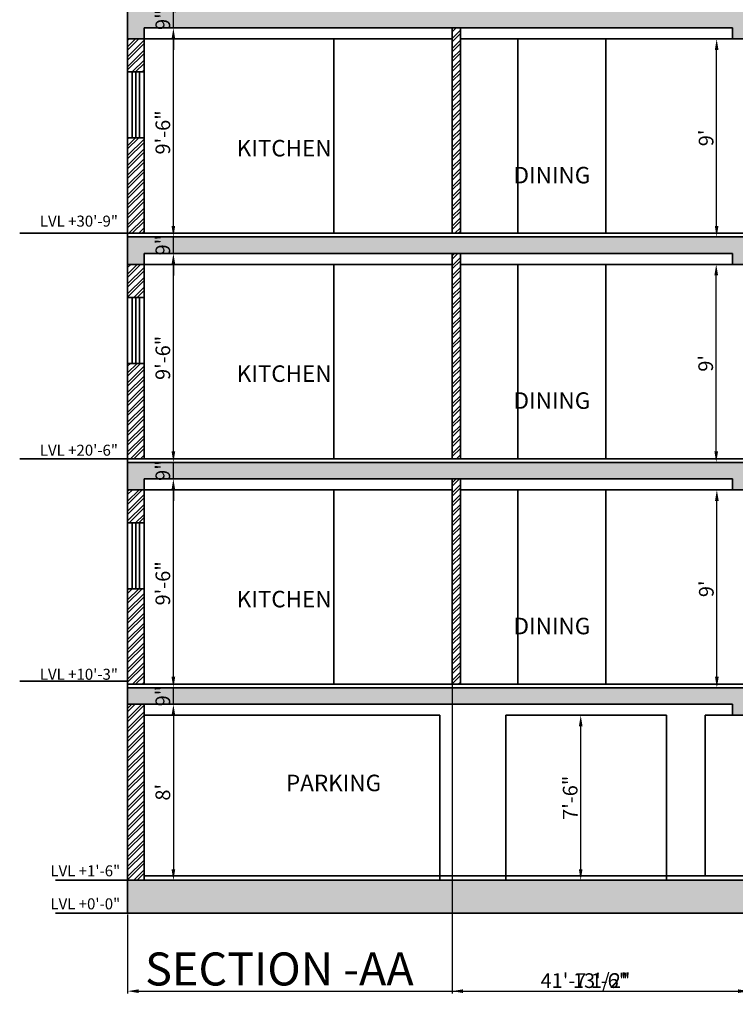
# Model space of a CAD drawing. Units: millimetres. Extents: x 1706 to 5913, y 156 to 1716.
# Tile 18 of 26: x 4417 to 4807, y 156 to 693. Entities that reach past the tile are written whole.
import ezdxf

# ---------------------------------------------------------------- set-up
doc = ezdxf.new("R2010")
doc.units = ezdxf.units.MM
for name, color, linetype, lineweight in [('A-ANNO-DIMS', 2, 'Continuous', 18), ('A-ANNO-SYMB', 3, 'Continuous', 18), ('A-ANNO-TEXT', 7, 'Continuous', 18), ('A-AREA-IDEN', 3, 'Continuous', 18), ('A-SECT', 7, 'Continuous', 35), ('A-SECT-PATT', 8, 'Continuous', 13)]:
    doc.layers.add(name, color=color, linetype=linetype, lineweight=lineweight)
doc.styles.get("Standard").update_dxf_attribs({"font": 'arial.ttf'})
doc.dimstyles.new('ISO-25', dxfattribs={"dimtxt": 8, "dimasz": 6, "dimexe": 1.25, "dimexo": 0.625, "dimtad": 1, "dimdec": 0, "dimlunit": 3, "dimtxsty": 'Standard', "dimcen": 2.5, "dimadec": 0, "dimazin": 0, "dimtfac": 1, "dimtdec": 0, "dimtmove": 0, "dimatfit": 3, "dimfxl": 1, "dimarcsym": 0})
pattern_1 = [(45, (229.4607, 1496.8062), (-2.6940768, 2.6940768), []), (45, (231.2567, 1496.8062), (-2.6940768, 2.6940768), [])]
pattern_2 = [(50, (229.461, 1496.806), (14.574774, -1.275127), [1.524, -16.764]), (355, (229.46, 1496.806), (-2.819474, 15.284548), [1.2192, -13.411247]), (100.45144, (230.675, 1496.7), (11.7553, 14.00942), [1.2952, -14.24722]), (46.1842, (229.46, 1500.87), (21.68632, -3.363386), [2.286, -25.146]), (96.63556, (231.268, 1500.59), (18.99233, 19.79409), [1.9428, -21.37085]), (351.18415, (229.46, 1500.87), (18.99233, 19.79409), [1.8288, -20.11678]), (21, (231.493, 1499.854), (12.12915, -8.181216), [1.524, -16.764]), (326, (231.493, 1499.854), (4.94416, 14.735037), [1.2192, -13.4112]), (71.45144, (232.503, 1499.172), (17.073314, 6.55382), [1.2952, -14.247195]), (37.5, (229.4607, 1496.806), (0.247088, 6.764403), [0, -13.24864, 0, -13.6144, 0, -13.462]), (7.5, (229.461, 1496.806), (5.345573, 8.014446), [0, -7.76224, 0, -12.94384, 0, -5.1308]), (327.5, (224.9293, 1496.806), (10.8472476, -0.4582995), [0, -5.08, 0, -15.8496, 0, -21.0312]), (317.5, (222.897, 1496.806), (11.850335, 2.03412), [0, -6.604, 0, -10.52576, 0, -14.9352])]

# ---------------------------------------------------------------- blocks, each defined once
blk = doc.blocks.new('*D169')
at = {"layer": 'A-ANNO-DIMS', "color": 0, "lineweight": -2, "transparency": 16777216}
for p, q in [((4503.77, 319.75), (4499.62, 319.75)), ((4500.87, 313.75), (4500.87, 229.75)), ((4503.77, 223.75), (4499.62, 223.75))]:
    blk.add_line(p, q, dxfattribs=at)
at = {"layer": 'A-ANNO-DIMS', "color": 0, "transparency": 16777216}
for points in [[(4499.87, 313.75), (4501.87, 313.75), (4500.87, 319.75)], [(4499.87, 229.75), (4501.87, 229.75), (4500.87, 223.75)]]:
    blk.add_solid(points, dxfattribs=at)
at = {"layer": 'Defpoints', "color": 0, "transparency": 16777216}
for p in [(4504.4, 319.75), (4500.87, 223.75), (4504.4, 223.75)]:
    blk.add_point(p, dxfattribs=at)
at = {"layer": 'A-ANNO-DIMS', "color": 0, "transparency": 16777216, "insert": (4496.16, 271.75), "char_height": 8, "attachment_point": 5, "rotation": 90}
blk.add_mtext("8'", dxfattribs=at)
blk = doc.blocks.new('*D170')
at = {"layer": 'A-ANNO-DIMS', "color": 0, "lineweight": -2, "transparency": 16777216}
for p, q in [((4721.21, 313.75), (4724.32, 313.75)), ((4723.07, 229.75), (4723.07, 307.75)), ((4721.21, 223.75), (4724.32, 223.75))]:
    blk.add_line(p, q, dxfattribs=at)
at = {"layer": 'A-ANNO-DIMS', "color": 0, "transparency": 16777216}
for points in [[(4722.07, 307.75), (4724.07, 307.75), (4723.07, 313.75)], [(4722.07, 229.75), (4724.07, 229.75), (4723.07, 223.75)]]:
    blk.add_solid(points, dxfattribs=at)
at = {"layer": 'Defpoints', "color": 0, "transparency": 16777216}
for p in [(4720.58, 313.75), (4723.07, 313.75), (4720.58, 223.75)]:
    blk.add_point(p, dxfattribs=at)
at = {"layer": 'A-ANNO-DIMS', "color": 0, "transparency": 16777216, "insert": (4718.36, 268.75), "char_height": 8, "attachment_point": 5, "rotation": 90}
blk.add_mtext('7\'-6"', dxfattribs=at)
blk = doc.blocks.new('*D171')
at = {"layer": 'A-ANNO-DIMS', "color": 0, "lineweight": -2, "transparency": 16777216}
for p, q in [((4500.87, 334.75), (4500.87, 340.75)), ((4500.87, 319.75), (4500.87, 328.75)), ((4501.49, 328.75), (4502.12, 328.75)), ((4501.49, 319.75), (4502.12, 319.75)), ((4500.87, 313.75), (4500.87, 307.75))]:
    blk.add_line(p, q, dxfattribs=at)
at = {"layer": 'A-ANNO-DIMS', "color": 0, "transparency": 16777216}
for points in [[(4499.87, 334.75), (4501.87, 334.75), (4500.87, 328.75)], [(4499.87, 313.75), (4501.87, 313.75), (4500.87, 319.75)]]:
    blk.add_solid(points, dxfattribs=at)
at = {"layer": 'Defpoints', "color": 0, "transparency": 16777216}
for p in [(4500.87, 328.75), (4500.87, 328.75), (4500.87, 319.75)]:
    blk.add_point(p, dxfattribs=at)
at = {"layer": 'A-ANNO-DIMS', "color": 0, "transparency": 16777216, "insert": (4496.16, 324.25), "char_height": 8, "attachment_point": 5, "rotation": 90}
blk.add_mtext('9"', dxfattribs=at)
blk = doc.blocks.new('*D172')
at = {"layer": 'A-ANNO-DIMS', "color": 0, "lineweight": -2, "transparency": 16777216}
for p, q in [((4501.49, 442.75), (4502.12, 442.75)), ((4500.87, 334.75), (4500.87, 436.75)), ((4501.49, 328.75), (4502.12, 328.75))]:
    blk.add_line(p, q, dxfattribs=at)
at = {"layer": 'A-ANNO-DIMS', "color": 0, "transparency": 16777216}
for points in [[(4499.87, 436.75), (4501.87, 436.75), (4500.87, 442.75)], [(4499.87, 334.75), (4501.87, 334.75), (4500.87, 328.75)]]:
    blk.add_solid(points, dxfattribs=at)
at = {"layer": 'Defpoints', "color": 0, "transparency": 16777216}
for p in [(4500.87, 442.75), (4500.87, 442.75), (4500.87, 328.75)]:
    blk.add_point(p, dxfattribs=at)
at = {"layer": 'A-ANNO-DIMS', "color": 0, "transparency": 16777216, "insert": (4496.16, 385.75), "char_height": 8, "attachment_point": 5, "rotation": 90}
blk.add_mtext('9\'-6"', dxfattribs=at)
blk = doc.blocks.new('*D173')
at = {"layer": 'A-ANNO-DIMS', "color": 0, "lineweight": -2, "transparency": 16777216}
for p, q in [((4500.87, 457.75), (4500.87, 463.75)), ((4500.87, 442.75), (4500.87, 451.75)), ((4501.49, 451.75), (4502.12, 451.75)), ((4501.49, 442.75), (4502.12, 442.75)), ((4500.87, 436.75), (4500.87, 430.75))]:
    blk.add_line(p, q, dxfattribs=at)
at = {"layer": 'A-ANNO-DIMS', "color": 0, "transparency": 16777216}
for points in [[(4499.87, 457.75), (4501.87, 457.75), (4500.87, 451.75)], [(4499.87, 436.75), (4501.87, 436.75), (4500.87, 442.75)]]:
    blk.add_solid(points, dxfattribs=at)
at = {"layer": 'Defpoints', "color": 0, "transparency": 16777216}
for p in [(4500.87, 451.75), (4500.87, 451.75), (4500.87, 442.75)]:
    blk.add_point(p, dxfattribs=at)
at = {"layer": 'A-ANNO-DIMS', "color": 0, "transparency": 16777216, "insert": (4496.16, 447.25), "char_height": 8, "attachment_point": 5, "rotation": 90}
blk.add_mtext('9"', dxfattribs=at)
blk = doc.blocks.new('*D174')
at = {"layer": 'A-ANNO-DIMS', "color": 0, "lineweight": -2, "transparency": 16777216}
for p, q in [((4501.49, 565.75), (4502.12, 565.75)), ((4500.87, 457.75), (4500.87, 559.75)), ((4501.49, 451.75), (4502.12, 451.75))]:
    blk.add_line(p, q, dxfattribs=at)
at = {"layer": 'A-ANNO-DIMS', "color": 0, "transparency": 16777216}
for points in [[(4499.87, 559.75), (4501.87, 559.75), (4500.87, 565.75)], [(4499.87, 457.75), (4501.87, 457.75), (4500.87, 451.75)]]:
    blk.add_solid(points, dxfattribs=at)
at = {"layer": 'Defpoints', "color": 0, "transparency": 16777216}
for p in [(4500.87, 565.75), (4500.87, 565.75), (4500.87, 451.75)]:
    blk.add_point(p, dxfattribs=at)
at = {"layer": 'A-ANNO-DIMS', "color": 0, "transparency": 16777216, "insert": (4496.16, 508.75), "char_height": 8, "attachment_point": 5, "rotation": 90}
blk.add_mtext('9\'-6"', dxfattribs=at)
blk = doc.blocks.new('*D175')
at = {"layer": 'A-ANNO-DIMS', "color": 0, "lineweight": -2, "transparency": 16777216}
for p, q in [((4500.87, 580.75), (4500.87, 586.75)), ((4500.24, 574.75), (4499.62, 574.75)), ((4500.87, 565.75), (4500.87, 574.75)), ((4500.24, 565.75), (4499.62, 565.75)), ((4500.87, 559.75), (4500.87, 553.75))]:
    blk.add_line(p, q, dxfattribs=at)
at = {"layer": 'A-ANNO-DIMS', "color": 0, "transparency": 16777216}
for points in [[(4499.87, 580.75), (4501.87, 580.75), (4500.87, 574.75)], [(4499.87, 559.75), (4501.87, 559.75), (4500.87, 565.75)]]:
    blk.add_solid(points, dxfattribs=at)
at = {"layer": 'Defpoints', "color": 0, "transparency": 16777216}
for p in [(4500.87, 574.75), (4500.87, 574.75), (4500.87, 565.75)]:
    blk.add_point(p, dxfattribs=at)
at = {"layer": 'A-ANNO-DIMS', "color": 0, "transparency": 16777216, "insert": (4496.16, 570.25), "char_height": 8, "attachment_point": 5, "rotation": 90}
blk.add_mtext('9"', dxfattribs=at)
blk = doc.blocks.new('*D176')
at = {"layer": 'A-ANNO-DIMS', "color": 0, "lineweight": -2, "transparency": 16777216}
for p, q in [((4501.49, 688.75), (4502.12, 688.75)), ((4500.87, 580.75), (4500.87, 682.75)), ((4501.49, 574.75), (4502.12, 574.75))]:
    blk.add_line(p, q, dxfattribs=at)
at = {"layer": 'A-ANNO-DIMS', "color": 0, "transparency": 16777216}
for points in [[(4499.87, 682.75), (4501.87, 682.75), (4500.87, 688.75)], [(4499.87, 580.75), (4501.87, 580.75), (4500.87, 574.75)]]:
    blk.add_solid(points, dxfattribs=at)
at = {"layer": 'Defpoints', "color": 0, "transparency": 16777216}
for p in [(4500.87, 688.75), (4500.87, 688.75), (4500.87, 574.75)]:
    blk.add_point(p, dxfattribs=at)
at = {"layer": 'A-ANNO-DIMS', "color": 0, "transparency": 16777216, "insert": (4496.16, 631.75), "char_height": 8, "attachment_point": 5, "rotation": 90}
blk.add_mtext('9\'-6"', dxfattribs=at)
blk = doc.blocks.new('*D177')
at = {"layer": 'A-ANNO-DIMS', "color": 0, "lineweight": -2, "transparency": 16777216}
for p, q in [((4500.87, 703.75), (4500.87, 709.75)), ((4500.87, 688.75), (4500.87, 697.75)), ((4501.49, 697.75), (4502.12, 697.75)), ((4501.49, 688.75), (4502.12, 688.75)), ((4500.87, 682.75), (4500.87, 676.75))]:
    blk.add_line(p, q, dxfattribs=at)
at = {"layer": 'A-ANNO-DIMS', "color": 0, "transparency": 16777216}
for points in [[(4499.87, 703.75), (4501.87, 703.75), (4500.87, 697.75)], [(4499.87, 682.75), (4501.87, 682.75), (4500.87, 688.75)]]:
    blk.add_solid(points, dxfattribs=at)
at = {"layer": 'Defpoints', "color": 0, "transparency": 16777216}
for p in [(4500.87, 697.75), (4500.87, 697.75), (4500.87, 688.75)]:
    blk.add_point(p, dxfattribs=at)
at = {"layer": 'A-ANNO-DIMS', "color": 0, "transparency": 16777216, "insert": (4496.16, 693.25), "char_height": 8, "attachment_point": 5, "rotation": 90}
blk.add_mtext('9"', dxfattribs=at)
blk = doc.blocks.new('*D180')
at = {"layer": 'A-ANNO-DIMS', "color": 0, "lineweight": -2, "transparency": 16777216}
for p, q in [((4800.25, 436.75), (4796.09, 436.75)), ((4797.34, 334.75), (4797.34, 430.75)), ((4800.25, 328.75), (4796.09, 328.75))]:
    blk.add_line(p, q, dxfattribs=at)
at = {"layer": 'A-ANNO-DIMS', "color": 0, "transparency": 16777216}
for points in [[(4796.34, 430.75), (4798.34, 430.75), (4797.34, 436.75)], [(4796.34, 334.75), (4798.34, 334.75), (4797.34, 328.75)]]:
    blk.add_solid(points, dxfattribs=at)
at = {"layer": 'Defpoints', "color": 0, "transparency": 16777216}
for p in [(4797.34, 436.75), (4800.87, 436.75), (4800.87, 328.75)]:
    blk.add_point(p, dxfattribs=at)
at = {"layer": 'A-ANNO-DIMS', "color": 0, "transparency": 16777216, "insert": (4792.63, 382.75), "char_height": 8, "attachment_point": 5, "rotation": 90}
blk.add_mtext("9'", dxfattribs=at)
blk = doc.blocks.new('*D181')
at = {"layer": 'A-ANNO-DIMS', "color": 0, "lineweight": -2, "transparency": 16777216}
for p, q in [((4796.72, 559.75), (4795.74, 559.75)), ((4796.99, 457.75), (4796.99, 553.75)), ((4796.72, 451.75), (4795.74, 451.75))]:
    blk.add_line(p, q, dxfattribs=at)
at = {"layer": 'A-ANNO-DIMS', "color": 0, "transparency": 16777216}
for points in [[(4795.99, 553.75), (4797.99, 553.75), (4796.99, 559.75)], [(4795.99, 457.75), (4797.99, 457.75), (4796.99, 451.75)]]:
    blk.add_solid(points, dxfattribs=at)
at = {"layer": 'Defpoints', "color": 0, "transparency": 16777216}
for p in [(4796.99, 559.75), (4797.34, 559.75), (4797.34, 451.75)]:
    blk.add_point(p, dxfattribs=at)
at = {"layer": 'A-ANNO-DIMS', "color": 0, "transparency": 16777216, "insert": (4792.28, 505.75), "char_height": 8, "attachment_point": 5, "rotation": 90}
blk.add_mtext("9'", dxfattribs=at)
blk = doc.blocks.new('*D182')
at = {"layer": 'A-ANNO-DIMS', "color": 0, "lineweight": -2, "transparency": 16777216}
for p, q in [((4797.62, 682.75), (4798.48, 682.75)), ((4797.23, 580.75), (4797.23, 676.75)), ((4797.62, 574.75), (4798.48, 574.75))]:
    blk.add_line(p, q, dxfattribs=at)
at = {"layer": 'A-ANNO-DIMS', "color": 0, "transparency": 16777216}
for points in [[(4796.23, 676.75), (4798.23, 676.75), (4797.23, 682.75)], [(4796.23, 580.75), (4798.23, 580.75), (4797.23, 574.75)]]:
    blk.add_solid(points, dxfattribs=at)
at = {"layer": 'Defpoints', "color": 0, "transparency": 16777216}
for p in [(4796.99, 682.75), (4797.23, 682.75), (4796.99, 574.75)]:
    blk.add_point(p, dxfattribs=at)
at = {"layer": 'A-ANNO-DIMS', "color": 0, "transparency": 16777216, "insert": (4792.52, 628.75), "char_height": 8, "attachment_point": 5, "rotation": 90}
blk.add_mtext("9'", dxfattribs=at)
blk = doc.blocks.new('*D250')
at = {"layer": 'A-ANNO-DIMS', "color": 0, "lineweight": -2, "transparency": 16777216}
for p, q in [((4475.91, 205.12), (4475.91, 162)), ((4975.41, 205.12), (4975.41, 162)), ((4481.91, 163.25), (4969.41, 163.25))]:
    blk.add_line(p, q, dxfattribs=at)
at = {"layer": 'A-ANNO-DIMS', "color": 0, "transparency": 16777216}
for points in [[(4481.91, 164.25), (4481.91, 162.25), (4475.91, 163.25)], [(4969.41, 164.25), (4969.41, 162.25), (4975.41, 163.25)]]:
    blk.add_solid(points, dxfattribs=at)
at = {"layer": 'Defpoints', "color": 0, "transparency": 16777216}
for p in [(4475.91, 205.75), (4975.41, 205.75), (4975.41, 163.25)]:
    blk.add_point(p, dxfattribs=at)
at = {"layer": 'A-ANNO-DIMS', "color": 0, "transparency": 16777216, "insert": (4725.66, 168.01), "char_height": 8, "attachment_point": 5}
blk.add_mtext('41\'-7 1/2"', dxfattribs=at)
blk = doc.blocks.new('*D254')
at = {"layer": 'A-ANNO-DIMS', "color": 0, "lineweight": -2, "transparency": 16777216}
for p, q in [((4652.91, 330.12), (4652.91, 162)), ((4814.91, 225.62), (4814.91, 162)), ((4658.91, 163.25), (4808.91, 163.25))]:
    blk.add_line(p, q, dxfattribs=at)
at = {"layer": 'A-ANNO-DIMS', "color": 0, "transparency": 16777216}
for points in [[(4658.91, 164.25), (4658.91, 162.25), (4652.91, 163.25)], [(4808.91, 164.25), (4808.91, 162.25), (4814.91, 163.25)]]:
    blk.add_solid(points, dxfattribs=at)
at = {"layer": 'Defpoints', "color": 0, "transparency": 16777216}
for p in [(4652.91, 330.75), (4814.91, 226.25), (4814.91, 163.25)]:
    blk.add_point(p, dxfattribs=at)
at = {"layer": 'A-ANNO-DIMS', "color": 0, "transparency": 16777216, "insert": (4733.91, 167.96), "char_height": 8, "attachment_point": 5}
blk.add_mtext('13\'-6"', dxfattribs=at)

msp = doc.modelspace()

# ---------------------------------------------------------------- hatches: boundary and pattern name
at = {"layer": 'A-SECT-PATT'}
h = msp.add_hatch(dxfattribs=at)
h.set_pattern_fill('AR-CONC', color=256, scale=0.08)
h.set_pattern_definition(pattern_2)
h.paths.add_polyline_path([(4853.91, 697.75), (4475.91, 697.75), (4475.91, 682.75), (4484.91, 682.75), (4484.91, 688.75), (4805.91, 688.75), (4805.91, 682.75), (4822.41, 682.75), (4822.41, 688.75), (4839.28, 688.75), (4927.41, 634.19), (4927.41, 634.75), (4966.41, 634.75), (4966.41, 632.75), (4975.41, 632.75), (4975.41, 641.25), (4927.41, 641.25), (4927.41, 647.75), (4916.91, 647.75), (4916.91, 654.25), (4906.41, 654.25), (4906.41, 660.75), (4895.91, 660.75), (4895.91, 667.25), (4885.41, 667.25), (4885.41, 673.75), (4874.91, 673.75), (4874.91, 680.25), (4864.41, 680.25), (4864.41, 686.75), (4853.91, 686.75)])
h = msp.add_hatch(dxfattribs=at)
h.set_pattern_fill('ANSI32', color=256, scale=0.4)
h.set_pattern_definition(pattern_1)
h.paths.add_polyline_path([(4657.41, 688.75), (4652.91, 688.75), (4652.91, 576.75), (4657.41, 576.75)])
h = msp.add_hatch(dxfattribs=at)
h.set_pattern_fill('ANSI32', color=256, scale=0.4)
h.set_pattern_definition(pattern_1)
h.paths.add_polyline_path([(4484.91, 682.75), (4475.91, 682.75), (4475.91, 664.75), (4484.91, 664.75)])
h = msp.add_hatch(dxfattribs=at)
h.set_pattern_fill('ANSI32', color=256, scale=0.4)
h.set_pattern_definition(pattern_1)
h.paths.add_polyline_path([(4484.91, 628.75), (4475.91, 628.75), (4475.91, 576.75), (4484.91, 576.75)])
h = msp.add_hatch(dxfattribs=at)
h.set_pattern_fill('AR-CONC', color=256, scale=0.08)
h.set_pattern_definition(pattern_2)
h.paths.add_polyline_path([(4853.91, 569.75), (4853.91, 574.75), (4475.91, 574.75), (4475.91, 559.75), (4484.91, 559.75), (4484.91, 565.75), (4805.91, 565.75), (4805.91, 559.75), (4822.41, 559.75), (4822.41, 565.75), (4838.47, 565.75), (4927.41, 510.69), (4927.41, 511.75), (4966.41, 511.75), (4966.41, 509.75), (4975.41, 509.75), (4975.41, 517.75), (4927.41, 517.75), (4927.41, 524.25), (4916.91, 524.25), (4916.91, 530.75), (4906.41, 530.75), (4906.41, 537.25), (4895.91, 537.25), (4895.91, 543.75), (4885.41, 543.75), (4885.41, 550.25), (4874.91, 550.25), (4874.91, 556.75), (4864.41, 556.75), (4864.41, 563.25), (4853.91, 563.25)])
h = msp.add_hatch(dxfattribs=at)
h.set_pattern_fill('ANSI32', color=256, scale=0.4)
h.set_pattern_definition(pattern_1)
h.paths.add_polyline_path([(4657.41, 565.75), (4652.91, 565.75), (4652.91, 453.75), (4657.41, 453.75)])
h = msp.add_hatch(dxfattribs=at)
h.set_pattern_fill('ANSI32', color=256, scale=0.4)
h.set_pattern_definition(pattern_1)
h.paths.add_polyline_path([(4484.91, 559.75), (4475.91, 559.75), (4475.91, 541.75), (4484.91, 541.75)])
h = msp.add_hatch(dxfattribs=at)
h.set_pattern_fill('ANSI32', color=256, scale=0.4)
h.set_pattern_definition(pattern_1)
h.paths.add_polyline_path([(4484.91, 505.75), (4475.91, 505.75), (4475.91, 453.75), (4484.91, 453.75)], flags=17)
h = msp.add_hatch(dxfattribs=at)
h.set_pattern_fill('AR-CONC', color=256, scale=0.08)
h.set_pattern_definition(pattern_2)
h.paths.add_polyline_path([(4853.91, 451.75), (4475.91, 451.75), (4475.91, 436.75), (4484.91, 436.75), (4484.91, 442.75), (4805.91, 442.75), (4805.91, 436.75), (4822.41, 436.75), (4822.41, 442.75), (4842.6, 442.75), (4927.41, 390.25), (4966.41, 390.25), (4966.41, 388.25), (4975.41, 388.25), (4975.41, 396.25), (4927.41, 396.25), (4927.41, 402.75), (4916.91, 402.75), (4916.91, 409.25), (4906.41, 409.25), (4906.41, 415.75), (4895.91, 415.75), (4895.91, 422.25), (4885.41, 422.25), (4885.41, 428.75), (4874.91, 428.75), (4874.91, 435.25), (4864.41, 435.25), (4864.41, 441.75), (4853.91, 441.75)])
h = msp.add_hatch(dxfattribs=at)
h.set_pattern_fill('ANSI32', color=256, scale=0.4)
h.set_pattern_definition(pattern_1)
h.paths.add_polyline_path([(4657.41, 442.75), (4652.91, 442.75), (4652.91, 330.75), (4657.41, 330.75)])
h = msp.add_hatch(dxfattribs=at)
h.set_pattern_fill('ANSI32', color=256, scale=0.4)
h.set_pattern_definition(pattern_1)
h.paths.add_polyline_path([(4484.91, 436.75), (4475.91, 436.75), (4475.91, 418.75), (4484.91, 418.75)])
h = msp.add_hatch(dxfattribs=at)
h.set_pattern_fill('ANSI32', color=256, scale=0.4)
h.set_pattern_definition(pattern_1)
h.paths.add_polyline_path([(4484.91, 382.75), (4475.91, 382.75), (4475.91, 330.75), (4484.91, 330.75)])
h = msp.add_hatch(dxfattribs=at)
h.set_pattern_fill('AR-CONC', color=256, scale=0.08)
h.set_pattern_definition(pattern_2)
h.paths.add_polyline_path([(4864.41, 323.25), (4853.91, 323.25), (4853.91, 328.75), (4475.91, 328.75), (4475.91, 319.75), (4805.91, 319.75), (4805.91, 313.75), (4814.91, 313.75), (4822.41, 313.75), (4822.41, 319.75), (4850.55, 319.75), (4927.41, 271.75), (4969.41, 271.75), (4969.41, 269.75), (4975.41, 269.75), (4975.41, 277.75), (4927.41, 277.75), (4927.41, 284.25), (4916.91, 284.25), (4916.91, 290.75), (4906.41, 290.75), (4906.41, 297.25), (4895.91, 297.25), (4895.91, 303.75), (4885.41, 303.75), (4885.41, 310.25), (4874.91, 310.25), (4874.91, 316.75), (4864.41, 316.75)])
h = msp.add_hatch(dxfattribs=at)
h.set_pattern_fill('ANSI32', color=256, scale=0.4)
h.set_pattern_definition(pattern_1)
h.paths.add_polyline_path([(4484.91, 319.75), (4475.91, 319.75), (4475.91, 223.75), (4484.91, 223.75)])
h = msp.add_hatch(dxfattribs=at)
h.set_pattern_fill('AR-CONC', color=256, scale=0.08)
h.set_pattern_definition(pattern_2)
h.paths.add_polyline_path([(4975.41, 223.75), (4475.91, 223.75), (4475.91, 205.75), (4975.41, 205.75)])

# ---------------------------------------------------------------- linework, layer by layer
at = {"layer": 'A-SECT'}
for p, q in [((4475.91, 856.75), (4475.91, 205.75)), ((4484.91, 688.75), (4484.91, 576.75)), ((4484.91, 688.75), (4805.91, 688.75)), ((4652.91, 688.75), (4652.91, 576.75)), ((4657.41, 688.75), (4657.41, 576.75)), ((4805.91, 682.75), (4805.91, 688.75)), ((4475.91, 682.75), (4652.91, 682.75)), ((4588.41, 682.75), (4588.41, 576.75)), ((4657.41, 682.75), (4822.41, 682.75)), ((4688.69, 576.75), (4688.69, 682.75)), ((4736.69, 576.75), (4736.69, 682.75)), ((4475.91, 664.75), (4484.91, 664.75)), ((4478.41, 664.75), (4478.41, 628.75)), ((4480.41, 664.75), (4480.41, 628.75)), ((4482.41, 664.75), (4482.41, 628.75)), ((4475.91, 628.75), (4484.91, 628.75)), ((4475.91, 576.75), (4417.04, 576.75)), ((4475.91, 574.75), (4853.91, 574.75)), ((4484.91, 565.75), (4484.91, 453.75)), ((4484.91, 565.75), (4805.91, 565.75)), ((4652.91, 565.75), (4652.91, 453.75)), ((4657.41, 565.75), (4657.41, 453.75)), ((4805.91, 559.75), (4805.91, 565.75)), ((4475.91, 559.75), (4652.91, 559.75)), ((4588.41, 559.75), (4588.41, 453.75)), ((4657.41, 559.75), (4822.41, 559.75)), ((4688.69, 453.75), (4688.69, 559.75)), ((4736.69, 453.75), (4736.69, 559.75)), ((4475.91, 541.75), (4484.91, 541.75)), ((4478.41, 541.75), (4478.41, 505.75)), ((4480.41, 541.75), (4480.41, 505.75)), ((4482.41, 541.75), (4482.41, 505.75)), ((4475.91, 505.75), (4484.91, 505.75)), ((4475.91, 453.75), (4417.04, 453.75)), ((4475.91, 451.75), (4853.91, 451.75)), ((4484.91, 442.75), (4484.91, 330.75)), ((4484.91, 442.75), (4805.91, 442.75)), ((4652.91, 442.75), (4652.91, 330.75)), ((4657.41, 442.75), (4657.41, 330.75)), ((4805.91, 436.75), (4805.91, 442.75)), ((4475.91, 436.75), (4652.91, 436.75)), ((4588.41, 436.75), (4588.41, 330.75)), ((4657.41, 436.75), (4822.41, 436.75)), ((4688.69, 330.75), (4688.69, 436.75)), ((4736.69, 330.75), (4736.69, 436.75)), ((4475.91, 418.75), (4484.91, 418.75)), ((4478.41, 418.75), (4478.41, 382.75)), ((4480.41, 418.75), (4480.41, 382.75)), ((4482.41, 418.75), (4482.41, 382.75)), ((4475.91, 382.75), (4484.91, 382.75)), ((4475.91, 332.33), (4417.04, 332.33)), ((4475.91, 328.75), (4853.91, 328.75)), ((4475.91, 319.75), (4805.91, 319.75)), ((4484.91, 319.75), (4484.91, 223.75)), ((4805.91, 319.75), (4805.91, 313.75)), ((4484.91, 313.75), (4646.18, 313.75)), ((4646.18, 313.75), (4646.18, 223.75)), ((4682.18, 313.75), (4682.18, 223.75)), ((4682.18, 313.75), (4769.96, 313.75)), ((4769.96, 313.75), (4769.96, 223.75)), ((4814.91, 313.75), (4790.91, 313.75)), ((4790.91, 313.75), (4790.91, 226.25)), ((4475.91, 223.75), (4436.57, 223.75)), ((4475.91, 223.75), (4975.41, 223.75)), ((4475.91, 205.75), (4436.57, 205.75)), ((4475.91, 205.75), (4975.41, 205.75))]:
    msp.add_line(p, q, dxfattribs=at)
for points in [[(4475.91, 664.75), (4484.91, 664.75), (4484.91, 628.75), (4475.91, 628.75)], [(4475.91, 541.75), (4484.91, 541.75), (4484.91, 505.75), (4475.91, 505.75)], [(4475.91, 418.75), (4484.91, 418.75), (4484.91, 382.75), (4475.91, 382.75)]]:
    msp.add_lwpolyline(points, close=True, dxfattribs=at)
for points in [[(4966.41, 519.75), (4929.41, 519.75), (4929.41, 526.25), (4918.91, 526.25), (4918.91, 532.75), (4908.41, 532.75), (4908.41, 539.25), (4897.91, 539.25), (4897.91, 545.75), (4887.41, 545.75), (4887.41, 552.25), (4876.91, 552.25), (4876.91, 558.75), (4866.41, 558.75), (4866.41, 565.25), (4855.91, 565.25), (4855.91, 569.75), (4855.91, 576.75), (4475.91, 576.75)], [(4966.41, 398.25), (4929.41, 398.25), (4929.41, 404.75), (4918.91, 404.75), (4918.91, 411.25), (4908.41, 411.25), (4908.41, 417.75), (4897.91, 417.75), (4897.91, 424.25), (4887.41, 424.25), (4887.41, 430.75), (4876.91, 430.75), (4876.91, 437.25), (4866.41, 437.25), (4866.41, 443.75), (4855.91, 443.75), (4855.91, 453.75), (4475.91, 453.75)], [(4929.41, 277.75), (4929.41, 286.25), (4918.91, 286.25), (4918.91, 292.75), (4908.41, 292.75), (4908.41, 299.25), (4897.91, 299.25), (4897.91, 305.75), (4887.41, 305.75), (4887.41, 312.25), (4876.91, 312.25), (4876.91, 318.75), (4866.41, 318.75), (4866.41, 325.25), (4855.91, 325.25), (4855.91, 330.75), (4475.91, 330.75)], [(4927.41, 271.75), (4927.41, 265.25), (4916.91, 265.25), (4916.91, 258.75), (4906.41, 258.75), (4906.41, 252.25), (4895.91, 252.25), (4895.91, 245.75), (4885.41, 245.75), (4885.41, 239.25), (4874.91, 239.25), (4874.91, 232.75), (4864.41, 232.75), (4864.41, 226.25), (4484.91, 226.25)]]:
    msp.add_lwpolyline(points, dxfattribs=at)

# ---------------------------------------------------------------- texts
at = {"layer": 'A-ANNO-SYMB', "char_height": 6, "attachment_point": 1}
for s, insert in [('      LVL +30\'-9"', (4417.04, 586.36)), ('      LVL +20\'-6"', (4417.04, 461.37)), ('      LVL +10\'-3"', (4417.04, 339.13)), ('      LVL +1\'-6"', (4422.8, 231.89)), ('      LVL +0\'-0"', (4422.8, 213.89))]:
    msp.add_mtext_dynamic_manual_height_columns(s, width=67.9131, gutter_width=12.5, heights=[0], dxfattribs=dict(at, insert=insert))
at = {"layer": 'A-ANNO-TEXT', "insert": (4479.95, 184.35), "char_height": 18, "attachment_point": 1}
msp.add_mtext_dynamic_manual_height_columns(' SECTION -AA', width=182.0755, gutter_width=12.5, heights=[0], dxfattribs=at)
at = {"layer": 'A-AREA-IDEN', "char_height": 9, "attachment_point": 1}
for s, insert in [('     KITCHEN', (4521.66, 627.65)), ('     DINING', (4672.68, 612.95)), ('     KITCHEN', (4521.66, 504.65)), ('     DINING', (4672.68, 489.95)), ('     KITCHEN', (4521.66, 381.65)), ('     DINING', (4672.68, 366.95)), ('     PARKING', (4548.53, 281.35))]:
    msp.add_mtext_dynamic_manual_height_columns(s, width=67.9131, gutter_width=12.5, heights=[0], dxfattribs=dict(at, insert=insert))

# ---------------------------------------------------------------- dimensions: what is measured, and where the dimension line sits
at = {"layer": 'A-ANNO-DIMS'}
for base, p1, p2, picture, middle in [((4500.87, 697.75), (4500.87, 688.75), (4500.87, 697.75), '*D177', (4500.87, 693.25)), ((4500.87, 574.75), (4500.87, 565.75), (4500.87, 574.75), '*D175', (4500.87, 570.25)), ((4500.87, 451.75), (4500.87, 442.75), (4500.87, 451.75), '*D173', (4500.87, 447.25)), ((4500.87, 328.75), (4500.87, 319.75), (4500.87, 328.75), '*D171', (4500.87, 324.25))]:
    dim = msp.add_linear_dim(base=base, p1=p1, p2=p2, angle=90, dimstyle='ISO-25', override={"dimclrd": 0, "dimclre": 0, "dimclrt": 0}, dxfattribs=at)
    dim.commit()
    dim.dimension.update_dxf_attribs({"geometry": picture, "text_midpoint": middle, "dimtype": 160})
for base, p1, p2, picture, middle in [((4500.87, 688.75), (4500.87, 574.75), (4500.87, 688.75), '*D176', (4496.16, 631.75)), ((4797.23, 682.75), (4796.99, 574.75), (4796.99, 682.75), '*D182', (4792.52, 628.75)), ((4500.87, 565.75), (4500.87, 451.75), (4500.87, 565.75), '*D174', (4496.16, 508.75)), ((4796.99, 559.75), (4797.34, 451.75), (4797.34, 559.75), '*D181', (4792.28, 505.75)), ((4500.87, 442.75), (4500.87, 328.75), (4500.87, 442.75), '*D172', (4496.16, 385.75)), ((4797.34, 436.75), (4800.87, 328.75), (4800.87, 436.75), '*D180', (4792.63, 382.75)), ((4500.87, 223.75), (4504.4, 319.75), (4504.4, 223.75), '*D169', (4496.16, 271.75)), ((4723.07, 313.75), (4720.58, 223.75), (4720.58, 313.75), '*D170', (4718.36, 268.75))]:
    dim = msp.add_linear_dim(base=base, p1=p1, p2=p2, angle=90, dimstyle='ISO-25', override={"dimclrd": 0, "dimclre": 0, "dimclrt": 0}, dxfattribs=at)
    dim.commit()
    dim.dimension.update_dxf_attribs({"geometry": picture, "text_midpoint": middle})
for base, p1, p2, picture, middle in [((4814.91, 163.25), (4652.91, 330.75), (4814.91, 226.25), '*D254', (4733.91, 167.96)), ((4975.41, 163.25), (4475.91, 205.75), (4975.41, 205.75), '*D250', (4725.66, 168.01))]:
    dim = msp.add_linear_dim(base=base, p1=p1, p2=p2, dimstyle='ISO-25', override={"dimdec": 1, "dimlfac": 1, "dimrnd": 0, "dimzin": 1, "dimdsep": 46, "dimlunit": 4, "dimfrac": 2}, dxfattribs=at)
    dim.commit()
    dim.dimension.update_dxf_attribs({"geometry": picture, "text_midpoint": middle})

doc.saveas('drawing.dxf')
